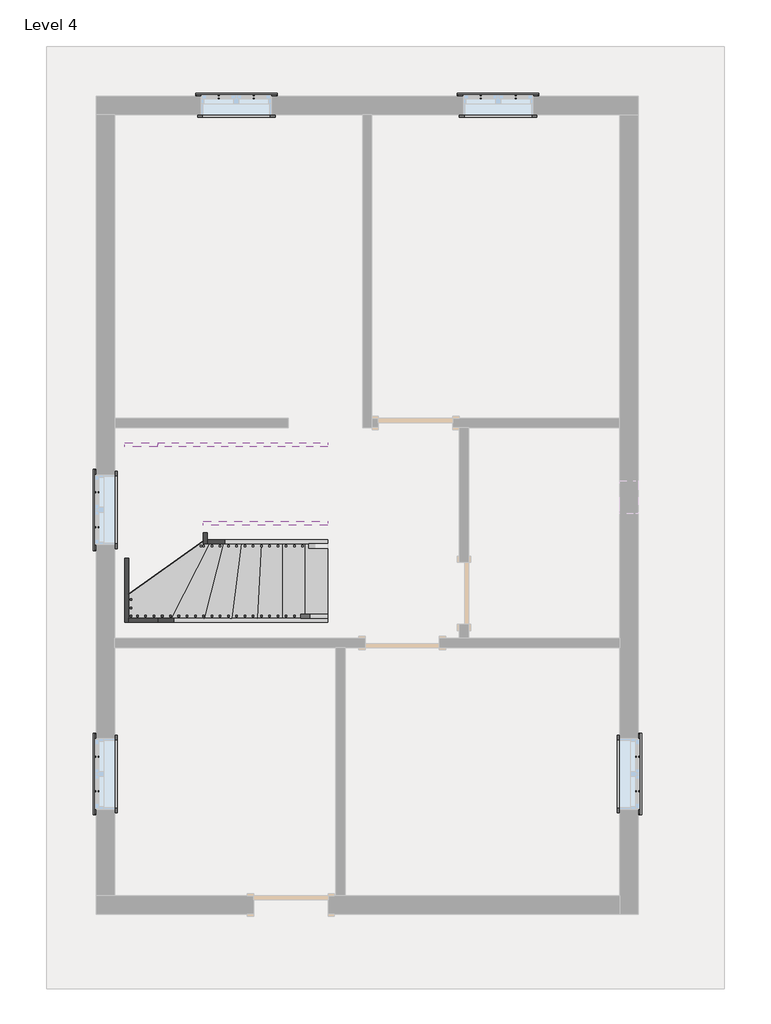
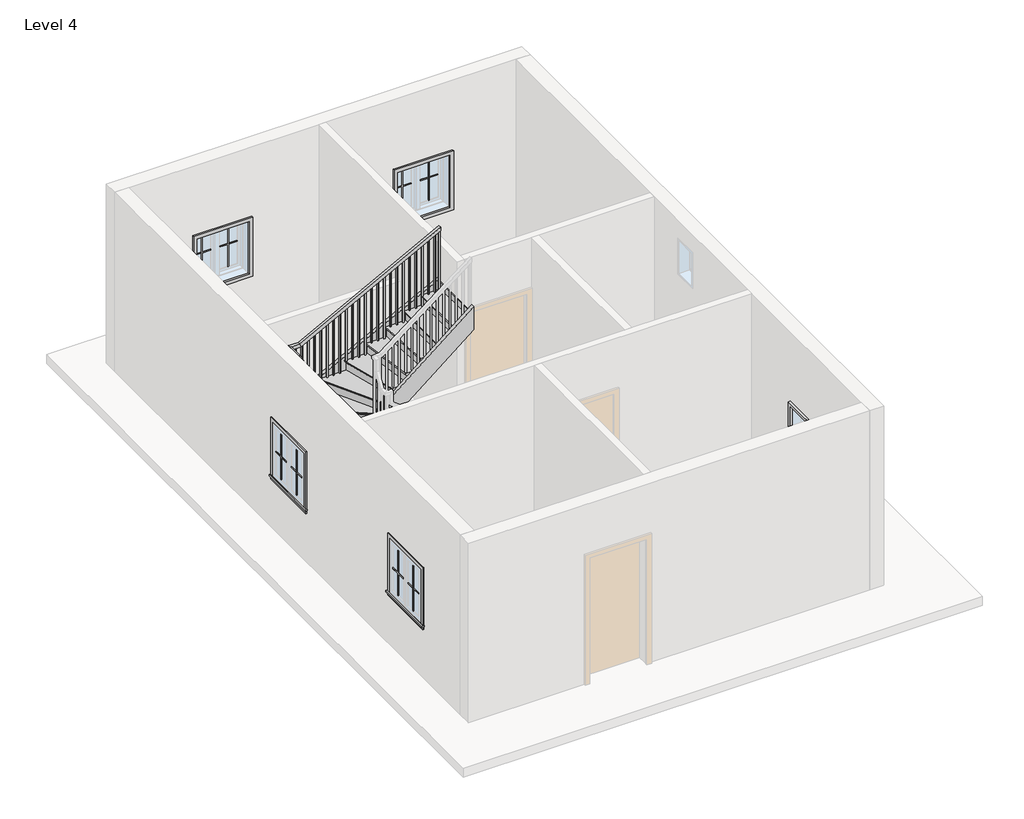
# One storey, part 2 of 2: 20 proxies, 8 members, 1 railing, 1 stair flight.
"""IFC4 building model written with IfcOpenShell, lengths in millimetres."""

from ifc_helpers import new_model, si_unit, frame, origin, place, context, project, spatial, polyline, outline, extrude, faceted_brep, transform, mapped, element, save
from components import muntin_pattern_2x2_muntin_pattern_2x2_b3fe6957, muntin_pattern_2x2_muntin_pattern_2x2_3e0ecaf2, trim_window_exterior_flat_with_sill_41619996, trim_window_interior_flat_picture_frame_51c85655, stair_flight_428a4bf9

model = new_model("IFC4")

# Units and contexts
model_context = context("Model", 3, world=origin())
ifc_project = project(units=[si_unit("LENGTHUNIT", "METRE", prefix="MILLI")], contexts=[model_context])

# Site, building, storey
site = spatial("IfcSite", under=ifc_project)
building = spatial("IfcBuilding", under=site)
storey = spatial("IfcBuildingStorey", under=building, Name="Level 4", Elevation=6400.8)

# Proxies
placement = place(None, origin())
muntin_pattern_2x2_muntin_pattern_2x2_shape = muntin_pattern_2x2_muntin_pattern_2x2_b3fe6957(model_context)
element("IfcBuildingElementProxy", 1, Name="Muntin Pattern_2x2 : Muntin Pattern_2x2", ObjectType="Muntin Pattern_2x2 : Muntin Pattern_2x2", at=placement, inside=storey, context=model_context, shape_type="MappedRepresentation", body=[
    mapped(muntin_pattern_2x2_muntin_pattern_2x2_shape, transform((-3096.8324167, 5150.2179147, 7385.05), x_axis=(1.0, 0.0, 0.0), y_axis=(0.0, 1.0, 0.0), z_axis=(0.0, 0.0, 1.0))),
])
element("IfcBuildingElementProxy", 2, Name="Muntin Pattern_2x2 : Muntin Pattern_2x2", ObjectType="Muntin Pattern_2x2 : Muntin Pattern_2x2", at=placement, inside=storey, context=model_context, shape_type="MappedRepresentation", body=[
    mapped(muntin_pattern_2x2_muntin_pattern_2x2_shape, transform((122.6175833, 5150.2179147, 7385.05), x_axis=(1.0, 0.0, 0.0), y_axis=(0.0, 1.0, 0.0), z_axis=(0.0, 0.0, 1.0))),
])
element("IfcBuildingElementProxy", 3, Name="Muntin Pattern_2x2 : Muntin Pattern_2x2", ObjectType="Muntin Pattern_2x2 : Muntin Pattern_2x2", at=placement, inside=storey, context=model_context, shape_type="MappedRepresentation", body=[
    mapped(muntin_pattern_2x2_muntin_pattern_2x2_shape, transform((-4597.0199167, -3388.9445853, 7385.05), x_axis=(0.0, 1.0, 0.0), y_axis=(-1.0, 0.0, 0.0), z_axis=(0.0, 0.0, 1.0))),
])
element("IfcBuildingElementProxy", 4, Name="Muntin Pattern_2x2 : Muntin Pattern_2x2", ObjectType="Muntin Pattern_2x2 : Muntin Pattern_2x2", at=placement, inside=storey, context=model_context, shape_type="MappedRepresentation", body=[
    mapped(muntin_pattern_2x2_muntin_pattern_2x2_shape, transform((2051.4300833, -2960.3195853, 7385.05), x_axis=(0.0, -1.0, 0.0), y_axis=(1.0, 0.0, 0.0), z_axis=(0.0, 0.0, 1.0))),
])
element("IfcBuildingElementProxy", 5, Name="Muntin Pattern_2x2 : Muntin Pattern_2x2", ObjectType="Muntin Pattern_2x2 : Muntin Pattern_2x2", at=placement, inside=storey, context=model_context, shape_type="MappedRepresentation", body=[
    mapped(muntin_pattern_2x2_muntin_pattern_2x2_shape, transform((-4597.0199167, -140.9195853, 7385.05), x_axis=(0.0, 1.0, 0.0), y_axis=(-1.0, 0.0, 0.0), z_axis=(0.0, 0.0, 1.0))),
])
muntin_pattern_2x2_muntin_pattern_2x2_2_shape = muntin_pattern_2x2_muntin_pattern_2x2_3e0ecaf2(model_context)
element("IfcBuildingElementProxy", 6, Name="Muntin Pattern_2x2 : Muntin Pattern_2x2", ObjectType="Muntin Pattern_2x2 : Muntin Pattern_2x2", at=placement, inside=storey, context=model_context, shape_type="MappedRepresentation", body=[
    mapped(muntin_pattern_2x2_muntin_pattern_2x2_2_shape, transform((-2668.2074167, 5150.2179147, 7385.05), x_axis=(-1.0, 0.0, 0.0), y_axis=(0.0, -1.0, 0.0), z_axis=(0.0, 0.0, 1.0))),
])
element("IfcBuildingElementProxy", 7, Name="Muntin Pattern_2x2 : Muntin Pattern_2x2", ObjectType="Muntin Pattern_2x2 : Muntin Pattern_2x2", at=placement, inside=storey, context=model_context, shape_type="MappedRepresentation", body=[
    mapped(muntin_pattern_2x2_muntin_pattern_2x2_2_shape, transform((551.2425833, 5150.2179147, 7385.05), x_axis=(-1.0, 0.0, 0.0), y_axis=(0.0, -1.0, 0.0), z_axis=(0.0, 0.0, 1.0))),
])
element("IfcBuildingElementProxy", 8, Name="Muntin Pattern_2x2 : Muntin Pattern_2x2", ObjectType="Muntin Pattern_2x2 : Muntin Pattern_2x2", at=placement, inside=storey, context=model_context, shape_type="MappedRepresentation", body=[
    mapped(muntin_pattern_2x2_muntin_pattern_2x2_2_shape, transform((-4597.0199167, -2960.3195853, 7385.05), x_axis=(0.0, -1.0, 0.0), y_axis=(1.0, 0.0, 0.0), z_axis=(0.0, 0.0, 1.0))),
])
element("IfcBuildingElementProxy", 9, Name="Muntin Pattern_2x2 : Muntin Pattern_2x2", ObjectType="Muntin Pattern_2x2 : Muntin Pattern_2x2", at=placement, inside=storey, context=model_context, shape_type="MappedRepresentation", body=[
    mapped(muntin_pattern_2x2_muntin_pattern_2x2_2_shape, transform((2051.4300833, -3388.9445853, 7385.05), x_axis=(0.0, 1.0, 0.0), y_axis=(-1.0, 0.0, 0.0), z_axis=(0.0, 0.0, 1.0))),
])
element("IfcBuildingElementProxy", 10, Name="Muntin Pattern_2x2 : Muntin Pattern_2x2", ObjectType="Muntin Pattern_2x2 : Muntin Pattern_2x2", at=placement, inside=storey, context=model_context, shape_type="MappedRepresentation", body=[
    mapped(muntin_pattern_2x2_muntin_pattern_2x2_2_shape, transform((-4597.0199167, 287.7054147, 7385.05), x_axis=(0.0, -1.0, 0.0), y_axis=(1.0, 0.0, 0.0), z_axis=(0.0, 0.0, 1.0))),
])
trim_window_exterior_flat_with_sill_shape = trim_window_exterior_flat_with_sill_41619996(model_context)
element("IfcBuildingElementProxy", 11, Name="Trim-Window-Exterior-Flat : with Sill", ObjectType="Trim-Window-Exterior-Flat : with Sill", at=placement, inside=storey, context=model_context, shape_type="MappedRepresentation", body=[
    mapped(trim_window_exterior_flat_with_sill_shape, transform((-2882.5199167, 5159.7429147, 8229.6), x_axis=(-1.0, 0.0, 0.0), y_axis=(0.0, 0.0, 1.0), z_axis=(0.0, 1.0, 0.0))),
])
element("IfcBuildingElementProxy", 12, Name="Trim-Window-Exterior-Flat : with Sill", ObjectType="Trim-Window-Exterior-Flat : with Sill", at=placement, inside=storey, context=model_context, shape_type="MappedRepresentation", body=[
    mapped(trim_window_exterior_flat_with_sill_shape, transform((336.9300833, 5159.7429147, 8229.6), x_axis=(-1.0, 0.0, 0.0), y_axis=(0.0, 0.0, 1.0), z_axis=(0.0, 1.0, 0.0))),
])
element("IfcBuildingElementProxy", 13, Name="Trim-Window-Exterior-Flat : with Sill", ObjectType="Trim-Window-Exterior-Flat : with Sill", at=placement, inside=storey, context=model_context, shape_type="MappedRepresentation", body=[
    mapped(trim_window_exterior_flat_with_sill_shape, transform((-4606.5449167, -3174.6320853, 8229.6), x_axis=(0.0, -1.0, 0.0), y_axis=(0.0, 0.0, 1.0), z_axis=(-1.0, 0.0, 0.0))),
])
element("IfcBuildingElementProxy", 14, Name="Trim-Window-Exterior-Flat : with Sill", ObjectType="Trim-Window-Exterior-Flat : with Sill", at=placement, inside=storey, context=model_context, shape_type="MappedRepresentation", body=[
    mapped(trim_window_exterior_flat_with_sill_shape, transform((2060.9550833, -3174.6320853, 8229.6), x_axis=(0.0, 1.0, 0.0), y_axis=(0.0, 0.0, 1.0), z_axis=(1.0, 0.0, 0.0))),
])
element("IfcBuildingElementProxy", 15, Name="Trim-Window-Exterior-Flat : with Sill", ObjectType="Trim-Window-Exterior-Flat : with Sill", at=placement, inside=storey, context=model_context, shape_type="MappedRepresentation", body=[
    mapped(trim_window_exterior_flat_with_sill_shape, transform((-4606.5449167, 73.3929147, 8229.6), x_axis=(0.0, -1.0, 0.0), y_axis=(0.0, 0.0, 1.0), z_axis=(-1.0, 0.0, 0.0))),
])
trim_window_interior_flat_picture_frame_shape = trim_window_interior_flat_picture_frame_51c85655(model_context)
element("IfcBuildingElementProxy", 16, Name="Trim-Window-Interior-Flat : Picture Frame", ObjectType="Trim-Window-Interior-Flat : Picture Frame", at=placement, inside=storey, context=model_context, shape_type="MappedRepresentation", body=[
    mapped(trim_window_interior_flat_picture_frame_shape, transform((-2882.5199167, 4931.1429147, 8229.6), x_axis=(1.0, 0.0, 0.0), y_axis=(0.0, 0.0, 1.0), z_axis=(0.0, -1.0, 0.0))),
])
element("IfcBuildingElementProxy", 17, Name="Trim-Window-Interior-Flat : Picture Frame", ObjectType="Trim-Window-Interior-Flat : Picture Frame", at=placement, inside=storey, context=model_context, shape_type="MappedRepresentation", body=[
    mapped(trim_window_interior_flat_picture_frame_shape, transform((336.9300833, 4931.1429147, 8229.6), x_axis=(1.0, 0.0, 0.0), y_axis=(0.0, 0.0, 1.0), z_axis=(0.0, -1.0, 0.0))),
])
element("IfcBuildingElementProxy", 18, Name="Trim-Window-Interior-Flat : Picture Frame", ObjectType="Trim-Window-Interior-Flat : Picture Frame", at=placement, inside=storey, context=model_context, shape_type="MappedRepresentation", body=[
    mapped(trim_window_interior_flat_picture_frame_shape, transform((-4377.9449167, -3174.6320853, 8229.6), x_axis=(0.0, 1.0, 0.0), y_axis=(0.0, 0.0, 1.0), z_axis=(1.0, 0.0, 0.0))),
])
element("IfcBuildingElementProxy", 19, Name="Trim-Window-Interior-Flat : Picture Frame", ObjectType="Trim-Window-Interior-Flat : Picture Frame", at=placement, inside=storey, context=model_context, shape_type="MappedRepresentation", body=[
    mapped(trim_window_interior_flat_picture_frame_shape, transform((1832.3550833, -3174.6320853, 8229.6), x_axis=(0.0, -1.0, 0.0), y_axis=(0.0, 0.0, 1.0), z_axis=(-1.0, 0.0, 0.0))),
])
element("IfcBuildingElementProxy", 20, Name="Trim-Window-Interior-Flat : Picture Frame", ObjectType="Trim-Window-Interior-Flat : Picture Frame", at=placement, inside=storey, context=model_context, shape_type="MappedRepresentation", body=[
    mapped(trim_window_interior_flat_picture_frame_shape, transform((-4377.9449167, 73.3929147, 8229.6), x_axis=(0.0, 1.0, 0.0), y_axis=(0.0, 0.0, 1.0), z_axis=(1.0, 0.0, 0.0))),
])

# Members
element("IfcMember", 21, ObjectType="Stringer - 2\" Width", at=placement, inside=storey, context=model_context, shape_type="SweptSolid", body=[
    extrude(outline(polyline([(6400.8, -1761.7449167), (6630.439954, -1761.7449167), (7706.1956453, -3849.1621084), (7363.300629, -3849.1621084), (6400.8, -1981.5072342), (6400.8, -1761.7449167)])), frame((0.0, -1310.9070853, 0.0), z_axis=(0.0, 1.0, 0.0), x_axis=(0.0, 0.0, 1.0)), (0.0, 0.0, 1.0), 50.8),
])
element("IfcMember", 22, ObjectType="Stringer - 2\" Width", at=placement, inside=storey, context=model_context, shape_type="SweptSolid", body=[
    extrude(outline(polyline([(-3849.1621084, -1260.1070853), (-3849.1621084, -1310.9070853), (-4203.8766085, -1310.9070853), (-4203.8766085, -1260.1070853), (-3849.1621084, -1260.1070853)])), frame((0.0, 0.0, 7363.300629), z_axis=(0.0, 0.0, 1.0), x_axis=(1.0, 0.0, 0.0)), (0.0, 0.0, 1.0), 342.8950162),
])
element("IfcMember", 23, ObjectType="Stringer - 2\" Width", at=placement, inside=storey, context=model_context, shape_type="SweptSolid", body=[
    extrude(outline(polyline([(-1310.9070853, 7401.3956453), (-1310.9070853, 7689.8952212), (811.1127974, 8370.7972697), (848.0929147, 8370.7972697), (848.0929147, 8039.7682298), (-1141.3846024, 7401.3956453), (-1310.9070853, 7401.3956453)])), frame((-4254.6766085, 0.0, 0.0), z_axis=(1.0, 0.0, 0.0), x_axis=(0.0, 1.0, 0.0)), (0.0, 0.0, 1.0), 50.8),
])
element("IfcMember", 24, ObjectType="Stringer - 2\" Width", at=placement, inside=storey, context=model_context, shape_type="SweptSolid", body=[
    extrude(outline(polyline([(-4254.6766085, 848.0929147), (-4254.6766085, 898.8929147), (-3849.1621084, 898.8929147), (-3849.1621084, 848.0929147), (-4254.6766085, 848.0929147)])), frame((0.0, 0.0, 8050.6904473), z_axis=(0.0, 0.0, 1.0), x_axis=(1.0, 0.0, 0.0)), (0.0, 0.0, 1.0), 320.1068224),
])
element("IfcMember", 25, ObjectType="Stringer - 2\" Width", at=placement, inside=storey, context=model_context, shape_type="SweptSolid", body=[
    extrude(outline(polyline([(8370.7972697, -3849.1621084), (8050.6904473, -3849.1621084), (9126.4461385, -1761.7449167), (9446.5529609, -1761.7449167), (8370.7972697, -3849.1621084)])), frame((0.0, 848.0929147, 0.0), z_axis=(0.0, 1.0, 0.0), x_axis=(0.0, 0.0, 1.0)), (0.0, 0.0, 1.0), 50.8),
])
element("IfcMember", 26, ObjectType="Stringer - 2\" Width", at=placement, inside=storey, context=model_context, shape_type="SweptSolid", body=[
    extrude(outline(polyline([(6400.8, -1761.7449167), (6576.9764461, -1761.7449167), (7781.218648, -3238.6766085), (7387.9410923, -3238.6766085), (6400.8, -2028.0065612), (6400.8, -1761.7449167)])), frame((0.0, -345.7070853, 0.0), z_axis=(0.0, 1.0, 0.0), x_axis=(0.0, 0.0, 1.0)), (0.0, 0.0, 1.0), 50.8),
])
element("IfcMember", 27, ObjectType="Stringer - 2\" Width", at=placement, inside=storey, context=model_context, shape_type="SweptSolid", body=[
    extrude(outline(polyline([(-345.7070853, 7429.3617647), (-345.7070853, 7974.0682978), (-139.0699679, 8326.9409689), (-117.1070853, 8326.9409689), (-117.1070853, 7761.265107), (-311.464868, 7429.3617647), (-345.7070853, 7429.3617647)])), frame((-3289.4766085, 0.0, 0.0), z_axis=(1.0, 0.0, 0.0), x_axis=(0.0, 1.0, 0.0)), (0.0, 0.0, 1.0), 50.8),
])
element("IfcMember", 28, ObjectType="Stringer - 2\" Width", at=placement, inside=storey, context=model_context, shape_type="SweptSolid", body=[
    extrude(outline(polyline([(8326.9409689, -3289.4766085), (7933.6634131, -3289.4766085), (9179.3262875, -1761.7449167), (9572.6038432, -1761.7449167), (8326.9409689, -3289.4766085)])), frame((0.0, -117.1070853, 0.0), z_axis=(0.0, 1.0, 0.0), x_axis=(0.0, 0.0, 1.0)), (0.0, 0.0, 1.0), 50.8),
])

# Railing
element("IfcRailing", 29, ObjectType="Handrail - Rectangular", at=placement, inside=storey, context=model_context, shape_type="SolidModel", body=[
    faceted_brep([(-1761.7449167, -1260.1070853, 7484.5333333), (-1761.7449167, -1260.1070853, 7427.0742652), (-1761.7449167, -1209.3070853, 7427.0742652), (-1761.7449167, -1209.3070853, 7484.5333333), (-4019.4699787, -1260.1070853, 8677.8239201), (-4032.0690433, -1260.1070853, 8627.0239201), (-4032.0690433, -1209.3070853, 8627.0239201), (-4019.4699787, -1209.3070853, 8677.8239201), (-4203.8766085, -1260.1070853, 8677.8239201), (-4203.8766085, -1260.1070853, 8627.0239201), (-4153.0766085, -1209.3070853, 8627.0239201), (-4153.0766085, -1209.3070853, 8677.8239201), (-4203.8766085, -972.7952032, 8677.8239201), (-4203.8766085, -964.8446271, 8627.0239201), (-4153.0766085, -964.8446271, 8627.0239201), (-4153.0766085, -972.7952032, 8677.8239201), (-4203.8766085, 560.7810325, 9169.9094132), (-4203.8766085, 568.7316087, 9119.1094132), (-4153.0766085, 568.7316087, 9119.1094132), (-4153.0766085, 560.7810325, 9169.9094132), (-4203.8766085, 848.0929147, 9169.9094132), (-4203.8766085, 848.0929147, 9119.1094132), (-4153.0766085, 797.2929147, 9119.1094132), (-4153.0766085, 797.2929147, 9169.9094132), (-4019.4699787, 848.0929147, 9169.9094132), (-4006.8709142, 848.0929147, 9119.1094132), (-4006.8709142, 797.2929147, 9119.1094132), (-4019.4699787, 797.2929147, 9169.9094132), (-1761.7449167, 848.0929147, 10363.2), (-1761.7449167, 797.2929147, 10363.2), (-1761.7449167, 797.2929147, 10305.7409318), (-1761.7449167, 848.0929147, 10305.7409318)], [[[0, 1, 2, 3]], [[1, 0, 4, 5]], [[2, 1, 5, 6]], [[3, 2, 6, 7]], [[0, 3, 7, 4]], [[5, 4, 8, 9]], [[6, 5, 9, 10]], [[7, 6, 10, 11]], [[4, 7, 11, 8]], [[9, 8, 12, 13]], [[10, 9, 13, 14]], [[11, 10, 14, 15]], [[8, 11, 15, 12]], [[13, 12, 16, 17]], [[14, 13, 17, 18]], [[15, 14, 18, 19]], [[12, 15, 19, 16]], [[17, 16, 20, 21]], [[18, 17, 21, 22]], [[19, 18, 22, 23]], [[16, 19, 23, 20]], [[21, 20, 24, 25]], [[22, 21, 25, 26]], [[23, 22, 26, 27]], [[20, 23, 27, 24]], [[28, 29, 30, 31]], [[25, 24, 28, 31]], [[26, 25, 31, 30]], [[27, 26, 30, 29]], [[24, 27, 29, 28]]]),
    extrude(outline(polyline([(10258.4597858, -1851.2016085), (9279.4666667, -1851.2016085), (9279.4666667, -1832.1516085), (10268.5284102, -1832.1516085), (10258.4597858, -1851.2016085)])), frame((0.0, 813.1679147, 0.0), z_axis=(0.0, 1.0, 0.0), x_axis=(0.0, 0.0, 1.0)), (0.0, 0.0, 1.0), 19.05),
    extrude(outline(polyline([(10204.7604556, -1952.8016085), (9279.4666667, -1952.8016085), (9279.4666667, -1933.7516085), (10214.82908, -1933.7516085), (10204.7604556, -1952.8016085)])), frame((0.0, 813.1679147, 0.0), z_axis=(0.0, 1.0, 0.0), x_axis=(0.0, 0.0, 1.0)), (0.0, 0.0, 1.0), 19.05),
    extrude(outline(polyline([(10151.0611254, -2054.4016085), (9110.1333333, -2054.4016085), (9110.1333333, -2035.3516085), (10161.1297498, -2035.3516085), (10151.0611254, -2054.4016085)])), frame((0.0, 813.1679147, 0.0), z_axis=(0.0, 1.0, 0.0), x_axis=(0.0, 0.0, 1.0)), (0.0, 0.0, 1.0), 19.05),
    extrude(outline(polyline([(10097.3617952, -2156.0016085), (9110.1333333, -2156.0016085), (9110.1333333, -2136.9516085), (10107.4304196, -2136.9516085), (10097.3617952, -2156.0016085)])), frame((0.0, 813.1679147, 0.0), z_axis=(0.0, 1.0, 0.0), x_axis=(0.0, 0.0, 1.0)), (0.0, 0.0, 1.0), 19.05),
    extrude(outline(polyline([(10043.662465, -2257.6016085), (9110.1333333, -2257.6016085), (9110.1333333, -2238.5516085), (10053.7310894, -2238.5516085), (10043.662465, -2257.6016085)])), frame((0.0, 813.1679147, 0.0), z_axis=(0.0, 1.0, 0.0), x_axis=(0.0, 0.0, 1.0)), (0.0, 0.0, 1.0), 19.05),
    extrude(outline(polyline([(9989.9631348, -2359.2016085), (8940.8, -2359.2016085), (8940.8, -2340.1516085), (10000.0317592, -2340.1516085), (9989.9631348, -2359.2016085)])), frame((0.0, 813.1679147, 0.0), z_axis=(0.0, 1.0, 0.0), x_axis=(0.0, 0.0, 1.0)), (0.0, 0.0, 1.0), 19.05),
    extrude(outline(polyline([(9936.2638046, -2460.8016085), (8940.8, -2460.8016085), (8940.8, -2441.7516085), (9946.332429, -2441.7516085), (9936.2638046, -2460.8016085)])), frame((0.0, 813.1679147, 0.0), z_axis=(0.0, 1.0, 0.0), x_axis=(0.0, 0.0, 1.0)), (0.0, 0.0, 1.0), 19.05),
    extrude(outline(polyline([(9882.5644744, -2562.4016085), (8940.8, -2562.4016085), (8940.8, -2543.3516085), (9892.6330988, -2543.3516085), (9882.5644744, -2562.4016085)])), frame((0.0, 813.1679147, 0.0), z_axis=(0.0, 1.0, 0.0), x_axis=(0.0, 0.0, 1.0)), (0.0, 0.0, 1.0), 19.05),
    extrude(outline(polyline([(9828.8651442, -2664.0016085), (8771.4666667, -2664.0016085), (8771.4666667, -2644.9516085), (9838.9337686, -2644.9516085), (9828.8651442, -2664.0016085)])), frame((0.0, 813.1679147, 0.0), z_axis=(0.0, 1.0, 0.0), x_axis=(0.0, 0.0, 1.0)), (0.0, 0.0, 1.0), 19.05),
    extrude(outline(polyline([(9775.165814, -2765.6016085), (8771.4666667, -2765.6016085), (8771.4666667, -2746.5516085), (9785.2344384, -2746.5516085), (9775.165814, -2765.6016085)])), frame((0.0, 813.1679147, 0.0), z_axis=(0.0, 1.0, 0.0), x_axis=(0.0, 0.0, 1.0)), (0.0, 0.0, 1.0), 19.05),
    extrude(outline(polyline([(9721.4664838, -2867.2016085), (8771.4666667, -2867.2016085), (8771.4666667, -2848.1516085), (9731.5351082, -2848.1516085), (9721.4664838, -2867.2016085)])), frame((0.0, 813.1679147, 0.0), z_axis=(0.0, 1.0, 0.0), x_axis=(0.0, 0.0, 1.0)), (0.0, 0.0, 1.0), 19.05),
    extrude(outline(polyline([(9667.7671536, -2968.8016085), (8602.1333333, -2968.8016085), (8602.1333333, -2949.7516085), (9677.835778, -2949.7516085), (9667.7671536, -2968.8016085)])), frame((0.0, 813.1679147, 0.0), z_axis=(0.0, 1.0, 0.0), x_axis=(0.0, 0.0, 1.0)), (0.0, 0.0, 1.0), 19.05),
    extrude(outline(polyline([(9614.0678234, -3070.4016085), (8602.1333333, -3070.4016085), (8602.1333333, -3051.3516085), (9624.1364478, -3051.3516085), (9614.0678234, -3070.4016085)])), frame((0.0, 813.1679147, 0.0), z_axis=(0.0, 1.0, 0.0), x_axis=(0.0, 0.0, 1.0)), (0.0, 0.0, 1.0), 19.05),
    extrude(outline(polyline([(9560.3684932, -3172.0016085), (8602.1333333, -3172.0016085), (8602.1333333, -3152.9516085), (9570.4371176, -3152.9516085), (9560.3684932, -3172.0016085)])), frame((0.0, 813.1679147, 0.0), z_axis=(0.0, 1.0, 0.0), x_axis=(0.0, 0.0, 1.0)), (0.0, 0.0, 1.0), 19.05),
    extrude(outline(polyline([(9506.669163, -3273.6016085), (8602.1333333, -3273.6016085), (8602.1333333, -3254.5516085), (9516.7377874, -3254.5516085), (9506.669163, -3273.6016085)])), frame((0.0, 813.1679147, 0.0), z_axis=(0.0, 1.0, 0.0), x_axis=(0.0, 0.0, 1.0)), (0.0, 0.0, 1.0), 19.05),
    extrude(outline(polyline([(9452.9698328, -3375.2016085), (8432.8, -3375.2016085), (8432.8, -3356.1516085), (9463.0384572, -3356.1516085), (9452.9698328, -3375.2016085)])), frame((0.0, 813.1679147, 0.0), z_axis=(0.0, 1.0, 0.0), x_axis=(0.0, 0.0, 1.0)), (0.0, 0.0, 1.0), 19.05),
    extrude(outline(polyline([(9399.2705026, -3476.8016085), (8432.8, -3476.8016085), (8432.8, -3457.7516085), (9409.339127, -3457.7516085), (9399.2705026, -3476.8016085)])), frame((0.0, 813.1679147, 0.0), z_axis=(0.0, 1.0, 0.0), x_axis=(0.0, 0.0, 1.0)), (0.0, 0.0, 1.0), 19.05),
    extrude(outline(polyline([(9345.5711724, -3578.4016085), (8432.8, -3578.4016085), (8432.8, -3559.3516085), (9355.6397968, -3559.3516085), (9345.5711724, -3578.4016085)])), frame((0.0, 813.1679147, 0.0), z_axis=(0.0, 1.0, 0.0), x_axis=(0.0, 0.0, 1.0)), (0.0, 0.0, 1.0), 19.05),
    extrude(outline(polyline([(9291.8718422, -3680.0016085), (8432.8, -3680.0016085), (8432.8, -3660.9516085), (9301.9404666, -3660.9516085), (9291.8718422, -3680.0016085)])), frame((0.0, 813.1679147, 0.0), z_axis=(0.0, 1.0, 0.0), x_axis=(0.0, 0.0, 1.0)), (0.0, 0.0, 1.0), 19.05),
    extrude(outline(polyline([(9238.172512, -3781.6016085), (8263.4666667, -3781.6016085), (8263.4666667, -3762.5516085), (9248.2411364, -3762.5516085), (9238.172512, -3781.6016085)])), frame((0.0, 813.1679147, 0.0), z_axis=(0.0, 1.0, 0.0), x_axis=(0.0, 0.0, 1.0)), (0.0, 0.0, 1.0), 19.05),
    extrude(outline(polyline([(9184.4731818, -3883.2016085), (8263.4666667, -3883.2016085), (8263.4666667, -3864.1516085), (9194.5418062, -3864.1516085), (9184.4731818, -3883.2016085)])), frame((0.0, 813.1679147, 0.0), z_axis=(0.0, 1.0, 0.0), x_axis=(0.0, 0.0, 1.0)), (0.0, 0.0, 1.0), 19.05),
    extrude(outline(polyline([(9130.7738516, -3984.8016085), (8263.4666667, -3984.8016085), (8263.4666667, -3965.7516085), (9140.842476, -3965.7516085), (9130.7738516, -3984.8016085)])), frame((0.0, 813.1679147, 0.0), z_axis=(0.0, 1.0, 0.0), x_axis=(0.0, 0.0, 1.0)), (0.0, 0.0, 1.0), 19.05),
    extrude(outline(polyline([(-4086.4016085, 832.2179147), (-4067.3516085, 832.2179147), (-4067.3516085, 813.1679147), (-4086.4016085, 813.1679147), (-4086.4016085, 832.2179147)])), frame((0.0, 0.0, 8263.4666667), z_axis=(0.0, 0.0, 1.0), x_axis=(1.0, 0.0, 0.0)), (0.0, 0.0, 1.0), 855.6427466),
    extrude(outline(polyline([(-4188.0016085, 787.7679147), (-4188.0016085, 806.8179147), (-4168.9516085, 806.8179147), (-4168.9516085, 787.7679147), (-4188.0016085, 787.7679147)])), frame((0.0, 0.0, 8263.4666667), z_axis=(0.0, 0.0, 1.0), x_axis=(1.0, 0.0, 0.0)), (0.0, 0.0, 1.0), 855.6427466),
    extrude(outline(polyline([(-4188.0016085, 686.1679147), (-4188.0016085, 705.2179147), (-4168.9516085, 705.2179147), (-4168.9516085, 686.1679147), (-4188.0016085, 686.1679147)])), frame((0.0, 0.0, 8263.4666667), z_axis=(0.0, 0.0, 1.0), x_axis=(1.0, 0.0, 0.0)), (0.0, 0.0, 1.0), 855.6427466),
    extrude(outline(polyline([(-4188.0016085, 584.5679147), (-4188.0016085, 603.6179147), (-4168.9516085, 603.6179147), (-4168.9516085, 584.5679147), (-4188.0016085, 584.5679147)])), frame((0.0, 0.0, 8263.4666667), z_axis=(0.0, 0.0, 1.0), x_axis=(1.0, 0.0, 0.0)), (0.0, 0.0, 1.0), 855.6427466),
    extrude(outline(polyline([(502.0179147, 9097.7026907), (502.0179147, 8094.1333333), (482.9679147, 8094.1333333), (482.9679147, 9091.5900316), (502.0179147, 9097.7026907)])), frame((-4188.0016085, 0.0, 0.0), z_axis=(1.0, 0.0, 0.0), x_axis=(0.0, 1.0, 0.0)), (0.0, 0.0, 1.0), 19.05),
    extrude(outline(polyline([(400.4179147, 9065.1018425), (400.4179147, 8094.1333333), (381.3679147, 8094.1333333), (381.3679147, 9058.9891834), (400.4179147, 9065.1018425)])), frame((-4188.0016085, 0.0, 0.0), z_axis=(1.0, 0.0, 0.0), x_axis=(0.0, 1.0, 0.0)), (0.0, 0.0, 1.0), 19.05),
    extrude(outline(polyline([(298.8179147, 9032.5009942), (298.8179147, 8094.1333333), (279.7679147, 8094.1333333), (279.7679147, 9026.3883352), (298.8179147, 9032.5009942)])), frame((-4188.0016085, 0.0, 0.0), z_axis=(1.0, 0.0, 0.0), x_axis=(0.0, 1.0, 0.0)), (0.0, 0.0, 1.0), 19.05),
    extrude(outline(polyline([(197.2179147, 8999.900146), (197.2179147, 8094.1333333), (178.1679147, 8094.1333333), (178.1679147, 8993.787487), (197.2179147, 8999.900146)])), frame((-4188.0016085, 0.0, 0.0), z_axis=(1.0, 0.0, 0.0), x_axis=(0.0, 1.0, 0.0)), (0.0, 0.0, 1.0), 19.05),
    extrude(outline(polyline([(95.6179147, 8967.2992978), (95.6179147, 8094.1333333), (76.5679147, 8094.1333333), (76.5679147, 8961.1866387), (95.6179147, 8967.2992978)])), frame((-4188.0016085, 0.0, 0.0), z_axis=(1.0, 0.0, 0.0), x_axis=(0.0, 1.0, 0.0)), (0.0, 0.0, 1.0), 19.05),
    extrude(outline(polyline([(-5.9820853, 8934.6984495), (-5.9820853, 7924.8), (-25.0320853, 7924.8), (-25.0320853, 8928.5857905), (-5.9820853, 8934.6984495)])), frame((-4188.0016085, 0.0, 0.0), z_axis=(1.0, 0.0, 0.0), x_axis=(0.0, 1.0, 0.0)), (0.0, 0.0, 1.0), 19.05),
    extrude(outline(polyline([(-107.5820853, 8902.0976013), (-107.5820853, 7924.8), (-126.6320853, 7924.8), (-126.6320853, 8895.9849423), (-107.5820853, 8902.0976013)])), frame((-4188.0016085, 0.0, 0.0), z_axis=(1.0, 0.0, 0.0), x_axis=(0.0, 1.0, 0.0)), (0.0, 0.0, 1.0), 19.05),
    extrude(outline(polyline([(-209.1820853, 8869.4967531), (-209.1820853, 7924.8), (-228.2320853, 7924.8), (-228.2320853, 8863.3840941), (-209.1820853, 8869.4967531)])), frame((-4188.0016085, 0.0, 0.0), z_axis=(1.0, 0.0, 0.0), x_axis=(0.0, 1.0, 0.0)), (0.0, 0.0, 1.0), 19.05),
    extrude(outline(polyline([(-310.7820853, 8836.8959049), (-310.7820853, 7924.8), (-329.8320853, 7924.8), (-329.8320853, 8830.7832458), (-310.7820853, 8836.8959049)])), frame((-4188.0016085, 0.0, 0.0), z_axis=(1.0, 0.0, 0.0), x_axis=(0.0, 1.0, 0.0)), (0.0, 0.0, 1.0), 19.05),
    extrude(outline(polyline([(-412.3820853, 8804.2950566), (-412.3820853, 7924.8), (-431.4320853, 7924.8), (-431.4320853, 8798.1823976), (-412.3820853, 8804.2950566)])), frame((-4188.0016085, 0.0, 0.0), z_axis=(1.0, 0.0, 0.0), x_axis=(0.0, 1.0, 0.0)), (0.0, 0.0, 1.0), 19.05),
    extrude(outline(polyline([(-513.9820853, 8771.6942084), (-513.9820853, 7755.4666667), (-533.0320853, 7755.4666667), (-533.0320853, 8765.5815494), (-513.9820853, 8771.6942084)])), frame((-4188.0016085, 0.0, 0.0), z_axis=(1.0, 0.0, 0.0), x_axis=(0.0, 1.0, 0.0)), (0.0, 0.0, 1.0), 19.05),
    extrude(outline(polyline([(-615.5820853, 8739.0933602), (-615.5820853, 7755.4666667), (-634.6320853, 7755.4666667), (-634.6320853, 8732.9807011), (-615.5820853, 8739.0933602)])), frame((-4188.0016085, 0.0, 0.0), z_axis=(1.0, 0.0, 0.0), x_axis=(0.0, 1.0, 0.0)), (0.0, 0.0, 1.0), 19.05),
    extrude(outline(polyline([(-717.1820853, 8706.492512), (-717.1820853, 7755.4666667), (-736.2320853, 7755.4666667), (-736.2320853, 8700.3798529), (-717.1820853, 8706.492512)])), frame((-4188.0016085, 0.0, 0.0), z_axis=(1.0, 0.0, 0.0), x_axis=(0.0, 1.0, 0.0)), (0.0, 0.0, 1.0), 19.05),
    extrude(outline(polyline([(-818.7820853, 8673.8916637), (-818.7820853, 7755.4666667), (-837.8320853, 7755.4666667), (-837.8320853, 8667.7790047), (-818.7820853, 8673.8916637)])), frame((-4188.0016085, 0.0, 0.0), z_axis=(1.0, 0.0, 0.0), x_axis=(0.0, 1.0, 0.0)), (0.0, 0.0, 1.0), 19.05),
    extrude(outline(polyline([(-920.3820853, 8641.2908155), (-920.3820853, 7755.4666667), (-939.4320853, 7755.4666667), (-939.4320853, 8635.1781565), (-920.3820853, 8641.2908155)])), frame((-4188.0016085, 0.0, 0.0), z_axis=(1.0, 0.0, 0.0), x_axis=(0.0, 1.0, 0.0)), (0.0, 0.0, 1.0), 19.05),
    extrude(outline(polyline([(-4188.0016085, -1041.0320853), (-4188.0016085, -1021.9820853), (-4168.9516085, -1021.9820853), (-4168.9516085, -1041.0320853), (-4188.0016085, -1041.0320853)])), frame((0.0, 0.0, 7586.1333333), z_axis=(0.0, 0.0, 1.0), x_axis=(1.0, 0.0, 0.0)), (0.0, 0.0, 1.0), 1040.8905868),
    extrude(outline(polyline([(-4188.0016085, -1142.6320853), (-4188.0016085, -1123.5820853), (-4168.9516085, -1123.5820853), (-4168.9516085, -1142.6320853), (-4188.0016085, -1142.6320853)])), frame((0.0, 0.0, 7586.1333333), z_axis=(0.0, 0.0, 1.0), x_axis=(1.0, 0.0, 0.0)), (0.0, 0.0, 1.0), 1040.8905868),
    extrude(outline(polyline([(-4089.0199167, -1244.2320853), (-4108.0699167, -1244.2320853), (-4108.0699167, -1225.1820853), (-4089.0199167, -1225.1820853), (-4089.0199167, -1244.2320853)])), frame((0.0, 0.0, 7586.1333333), z_axis=(0.0, 0.0, 1.0), x_axis=(1.0, 0.0, 0.0)), (0.0, 0.0, 1.0), 1040.8905868),
    extrude(outline(polyline([(8613.4938418, -4006.4699167), (7586.1333333, -4006.4699167), (7586.1333333, -3987.4199167), (8603.4252174, -3987.4199167), (8613.4938418, -4006.4699167)])), frame((0.0, -1244.2320853, 0.0), z_axis=(0.0, 1.0, 0.0), x_axis=(0.0, 0.0, 1.0)), (0.0, 0.0, 1.0), 19.05),
    extrude(outline(polyline([(8559.7945116, -3904.8699167), (7586.1333333, -3904.8699167), (7586.1333333, -3885.8199167), (8549.7258872, -3885.8199167), (8559.7945116, -3904.8699167)])), frame((0.0, -1244.2320853, 0.0), z_axis=(0.0, 1.0, 0.0), x_axis=(0.0, 0.0, 1.0)), (0.0, 0.0, 1.0), 19.05),
    extrude(outline(polyline([(8506.0951814, -3803.2699167), (7586.1333333, -3803.2699167), (7586.1333333, -3784.2199167), (8496.026557, -3784.2199167), (8506.0951814, -3803.2699167)])), frame((0.0, -1244.2320853, 0.0), z_axis=(0.0, 1.0, 0.0), x_axis=(0.0, 0.0, 1.0)), (0.0, 0.0, 1.0), 19.05),
    extrude(outline(polyline([(8452.3958512, -3701.6699167), (7586.1333333, -3701.6699167), (7586.1333333, -3682.6199167), (8442.3272268, -3682.6199167), (8452.3958512, -3701.6699167)])), frame((0.0, -1244.2320853, 0.0), z_axis=(0.0, 1.0, 0.0), x_axis=(0.0, 0.0, 1.0)), (0.0, 0.0, 1.0), 19.05),
    extrude(outline(polyline([(8398.696521, -3600.0699167), (7416.8, -3600.0699167), (7416.8, -3581.0199167), (8388.6278966, -3581.0199167), (8398.696521, -3600.0699167)])), frame((0.0, -1244.2320853, 0.0), z_axis=(0.0, 1.0, 0.0), x_axis=(0.0, 0.0, 1.0)), (0.0, 0.0, 1.0), 19.05),
    extrude(outline(polyline([(8344.9971908, -3498.4699167), (7416.8, -3498.4699167), (7416.8, -3479.4199167), (8334.9285664, -3479.4199167), (8344.9971908, -3498.4699167)])), frame((0.0, -1244.2320853, 0.0), z_axis=(0.0, 1.0, 0.0), x_axis=(0.0, 0.0, 1.0)), (0.0, 0.0, 1.0), 19.05),
    extrude(outline(polyline([(8291.2978606, -3396.8699167), (7416.8, -3396.8699167), (7416.8, -3377.8199167), (8281.2292362, -3377.8199167), (8291.2978606, -3396.8699167)])), frame((0.0, -1244.2320853, 0.0), z_axis=(0.0, 1.0, 0.0), x_axis=(0.0, 0.0, 1.0)), (0.0, 0.0, 1.0), 19.05),
    extrude(outline(polyline([(8237.5985304, -3295.2699167), (7416.8, -3295.2699167), (7416.8, -3276.2199167), (8227.529906, -3276.2199167), (8237.5985304, -3295.2699167)])), frame((0.0, -1244.2320853, 0.0), z_axis=(0.0, 1.0, 0.0), x_axis=(0.0, 0.0, 1.0)), (0.0, 0.0, 1.0), 19.05),
    extrude(outline(polyline([(8183.8992002, -3193.6699167), (7247.4666667, -3193.6699167), (7247.4666667, -3174.6199167), (8173.8305758, -3174.6199167), (8183.8992002, -3193.6699167)])), frame((0.0, -1244.2320853, 0.0), z_axis=(0.0, 1.0, 0.0), x_axis=(0.0, 0.0, 1.0)), (0.0, 0.0, 1.0), 19.05),
    extrude(outline(polyline([(8130.19987, -3092.0699167), (7247.4666667, -3092.0699167), (7247.4666667, -3073.0199167), (8120.1312456, -3073.0199167), (8130.19987, -3092.0699167)])), frame((0.0, -1244.2320853, 0.0), z_axis=(0.0, 1.0, 0.0), x_axis=(0.0, 0.0, 1.0)), (0.0, 0.0, 1.0), 19.05),
    extrude(outline(polyline([(8076.5005398, -2990.4699167), (7247.4666667, -2990.4699167), (7247.4666667, -2971.4199167), (8066.4319154, -2971.4199167), (8076.5005398, -2990.4699167)])), frame((0.0, -1244.2320853, 0.0), z_axis=(0.0, 1.0, 0.0), x_axis=(0.0, 0.0, 1.0)), (0.0, 0.0, 1.0), 19.05),
    extrude(outline(polyline([(8022.8012096, -2888.8699167), (7078.1333333, -2888.8699167), (7078.1333333, -2869.8199167), (8012.7325852, -2869.8199167), (8022.8012096, -2888.8699167)])), frame((0.0, -1244.2320853, 0.0), z_axis=(0.0, 1.0, 0.0), x_axis=(0.0, 0.0, 1.0)), (0.0, 0.0, 1.0), 19.05),
    extrude(outline(polyline([(7969.1018794, -2787.2699167), (7078.1333333, -2787.2699167), (7078.1333333, -2768.2199167), (7959.033255, -2768.2199167), (7969.1018794, -2787.2699167)])), frame((0.0, -1244.2320853, 0.0), z_axis=(0.0, 1.0, 0.0), x_axis=(0.0, 0.0, 1.0)), (0.0, 0.0, 1.0), 19.05),
    extrude(outline(polyline([(7915.4025492, -2685.6699167), (7078.1333333, -2685.6699167), (7078.1333333, -2666.6199167), (7905.3339248, -2666.6199167), (7915.4025492, -2685.6699167)])), frame((0.0, -1244.2320853, 0.0), z_axis=(0.0, 1.0, 0.0), x_axis=(0.0, 0.0, 1.0)), (0.0, 0.0, 1.0), 19.05),
    extrude(outline(polyline([(7861.703219, -2584.0699167), (6908.8, -2584.0699167), (6908.8, -2565.0199167), (7851.6345946, -2565.0199167), (7861.703219, -2584.0699167)])), frame((0.0, -1244.2320853, 0.0), z_axis=(0.0, 1.0, 0.0), x_axis=(0.0, 0.0, 1.0)), (0.0, 0.0, 1.0), 19.05),
    extrude(outline(polyline([(7808.0038888, -2482.4699167), (6908.8, -2482.4699167), (6908.8, -2463.4199167), (7797.9352644, -2463.4199167), (7808.0038888, -2482.4699167)])), frame((0.0, -1244.2320853, 0.0), z_axis=(0.0, 1.0, 0.0), x_axis=(0.0, 0.0, 1.0)), (0.0, 0.0, 1.0), 19.05),
    extrude(outline(polyline([(7754.3045586, -2380.8699167), (6908.8, -2380.8699167), (6908.8, -2361.8199167), (7744.2359342, -2361.8199167), (7754.3045586, -2380.8699167)])), frame((0.0, -1244.2320853, 0.0), z_axis=(0.0, 1.0, 0.0), x_axis=(0.0, 0.0, 1.0)), (0.0, 0.0, 1.0), 19.05),
    extrude(outline(polyline([(7700.6052284, -2279.2699167), (6739.4666667, -2279.2699167), (6739.4666667, -2260.2199167), (7690.536604, -2260.2199167), (7700.6052284, -2279.2699167)])), frame((0.0, -1244.2320853, 0.0), z_axis=(0.0, 1.0, 0.0), x_axis=(0.0, 0.0, 1.0)), (0.0, 0.0, 1.0), 19.05),
    extrude(outline(polyline([(7646.9058982, -2177.6699167), (6739.4666667, -2177.6699167), (6739.4666667, -2158.6199167), (7636.8372738, -2158.6199167), (7646.9058982, -2177.6699167)])), frame((0.0, -1244.2320853, 0.0), z_axis=(0.0, 1.0, 0.0), x_axis=(0.0, 0.0, 1.0)), (0.0, 0.0, 1.0), 19.05),
    extrude(outline(polyline([(7593.206568, -2076.0699167), (6739.4666667, -2076.0699167), (6739.4666667, -2057.0199167), (7583.1379436, -2057.0199167), (7593.206568, -2076.0699167)])), frame((0.0, -1244.2320853, 0.0), z_axis=(0.0, 1.0, 0.0), x_axis=(0.0, 0.0, 1.0)), (0.0, 0.0, 1.0), 19.05),
    extrude(outline(polyline([(7539.5072378, -1974.4699167), (6570.1333333, -1974.4699167), (6570.1333333, -1955.4199167), (7529.4386134, -1955.4199167), (7539.5072378, -1974.4699167)])), frame((0.0, -1244.2320853, 0.0), z_axis=(0.0, 1.0, 0.0), x_axis=(0.0, 0.0, 1.0)), (0.0, 0.0, 1.0), 19.05),
    extrude(outline(polyline([(7485.8079076, -1872.8699167), (6570.1333333, -1872.8699167), (6570.1333333, -1853.8199167), (7475.7392831, -1853.8199167), (7485.8079076, -1872.8699167)])), frame((0.0, -1244.2320853, 0.0), z_axis=(0.0, 1.0, 0.0), x_axis=(0.0, 0.0, 1.0)), (0.0, 0.0, 1.0), 19.05),
    extrude(outline(polyline([(-4188.0016085, 813.1679147), (-4188.0016085, 832.2179147), (-4168.9516085, 832.2179147), (-4168.9516085, 813.1679147), (-4188.0016085, 813.1679147)])), frame((0.0, 0.0, 8263.4666667), z_axis=(0.0, 0.0, 1.0), x_axis=(1.0, 0.0, 0.0)), (0.0, 0.0, 1.0), 855.6427466),
    extrude(outline(polyline([(-4168.9516085, -1244.2320853), (-4188.0016085, -1244.2320853), (-4188.0016085, -1225.1820853), (-4168.9516085, -1225.1820853), (-4168.9516085, -1244.2320853)])), frame((0.0, 0.0, 7586.1333333), z_axis=(0.0, 0.0, 1.0), x_axis=(1.0, 0.0, 0.0)), (0.0, 0.0, 1.0), 1040.8905868),
    extrude(outline(polyline([(10295.6723074, -1780.7949167), (9279.4666667, -1780.7949167), (9279.4666667, -1761.7449167), (10305.7409318, -1761.7449167), (10295.6723074, -1780.7949167)])), frame((0.0, 813.1679147, 0.0), z_axis=(0.0, 1.0, 0.0), x_axis=(0.0, 0.0, 1.0)), (0.0, 0.0, 1.0), 19.05),
    extrude(outline(polyline([(7437.1428896, -1780.7949167), (6570.1333333, -1780.7949167), (6570.1333333, -1761.7449167), (7427.0742652, -1761.7449167), (7437.1428896, -1780.7949167)])), frame((0.0, -1244.2320853, 0.0), z_axis=(0.0, 1.0, 0.0), x_axis=(0.0, 0.0, 1.0)), (0.0, 0.0, 1.0), 19.05),
])

# Stair flight
stair_flight_shape = stair_flight_428a4bf9(model_context)
element("IfcStairFlight", 30, ObjectType="2\" Tread 1\" Nosing 1/4\" Riser", at=placement, inside=storey, context=model_context, shape_type="MappedRepresentation", body=[
    mapped(stair_flight_shape, transform((0.0, 0.0, 0.0), x_axis=(1.0, 0.0, 0.0), y_axis=(0.0, 1.0, 0.0), z_axis=(0.0, 0.0, 1.0))),
])

save(model, "model.ifc")

# Revit data of these elements
# Type "Muntin Pattern_2x2 : Muntin Pattern_2x2"
#   Width [instance default] = 4' - 0"
#   Thickness = 0' - 0 1/2"
#   Height [instance default] = 4' - 0"
#   Distance = 0' - 0 3/4"
#   Interior Material [instance default] = none
#   Exterior Material [instance default] = none
#   Default Elevation = 0
# Type "Trim-Window-Exterior-Flat : with Sill"
#   Trim Width = 0' - 2 1/4"
#   Trim Thickness_Picture Frame = 0' - 1 1/4"
#   Trim Thickness_with Sill = 0' - 0 3/4"
#   Sill Thickness = 0' - 1 1/4"
#   Opening Width [instance default] = 2' - 0"
#   Opening Height [instance default] = 3' - 0"
#   Default Elevation = 4' - 0"
#   Sill = yes
#   Picture Frame = no
#   Trim Material [instance default] = none
# Type "Trim-Window-Interior-Flat : Picture Frame"
#   Trim Thickness_Picture Frame = 0' - 1 1/4"
#   Trim Width = 0' - 2 1/4"
#   Trim Thickness_with Sill = 0' - 0 3/4"
#   Sill Thickness = 0' - 1 1/4"
#   Opening Width [instance default] = 2' - 0"
#   Opening Height [instance default] = 3' - 0"
#   Default Elevation = 4' - 0"
#   Sill = no
#   Picture Frame = yes
#   Trim Material [instance default] = none
# Type "Handrail - Rectangular"
#   Assembly Code = "C2010400"
#   built-in parameter 1008612 = 0.0416667 (stored number, unit not read)
#   built-in parameter 1008611 = 0.0416667 (stored number, unit not read)
#   built-in parameter 1008609 = 0.333333 (stored number, unit not read)
#   built-in parameter 1008604 = 0.166667 (stored number, unit not read)
#   built-in parameter 1008603 = 0.166667 (stored number, unit not read)
#   Railing Height = 3' - 0"
#   built-in parameter 1008630 = 2
#   built-in parameter 1008610 = 2
#   built-in parameter 1008618 = Baluster - Square : 3/4"
# Elements 1, 2, 3, 4, 5, 6, 7, 8, 9, 10 (IfcBuildingElementProxy, "Muntin Pattern_2x2 : Muntin Pattern_2x2")
#   Width = 0' - 11 5/8"
#   Height = 2' - 6 1/2"
#   Interior Material = Wood - Stained
#   Exterior Material = Clad - White
#   Phase Created = New Construction
#   Materials on its faces: "Clad - White", "Wood - Stained"
# Elements 11, 12, 13, 14, 15 (IfcBuildingElementProxy, "Trim-Window-Exterior-Flat : with Sill")
#   Opening Width = 2' - 10"
#   Opening Height = 3' - 0"
#   Trim Material = Clad - White
#   Phase Created = New Construction
#   Materials on its faces: "Clad - White"
# Elements 16, 17, 18, 19, 20 (IfcBuildingElementProxy, "Trim-Window-Interior-Flat : Picture Frame")
#   Opening Width = 2' - 10"
#   Opening Height = 3' - 0"
#   Trim Material = Wood - Stained
#   Phase Created = New Construction
#   Materials on its faces: "Wood - Stained"
# Elements 21, 22, 23, 24, 25, 26, 27, 28 (IfcMember, "Stringer - 2\" Width")
#   Phase Created = New Construction
# Element 29 (IfcRailing, "Handrail - Rectangular")
#   Phase Created = New Construction
# Element 30 (IfcStairFlight, "2\" Tread 1\" Nosing 1/4\" Riser")
#   Phase Created = New Construction
# Materials
#   "Clad - White": class "Wood", colour RGB 242 242 238, transparency 0, Cost = 0
#   "Wood - Stained": class "Wood", colour RGB 224 178 126, transparency 0, Cost = 0
